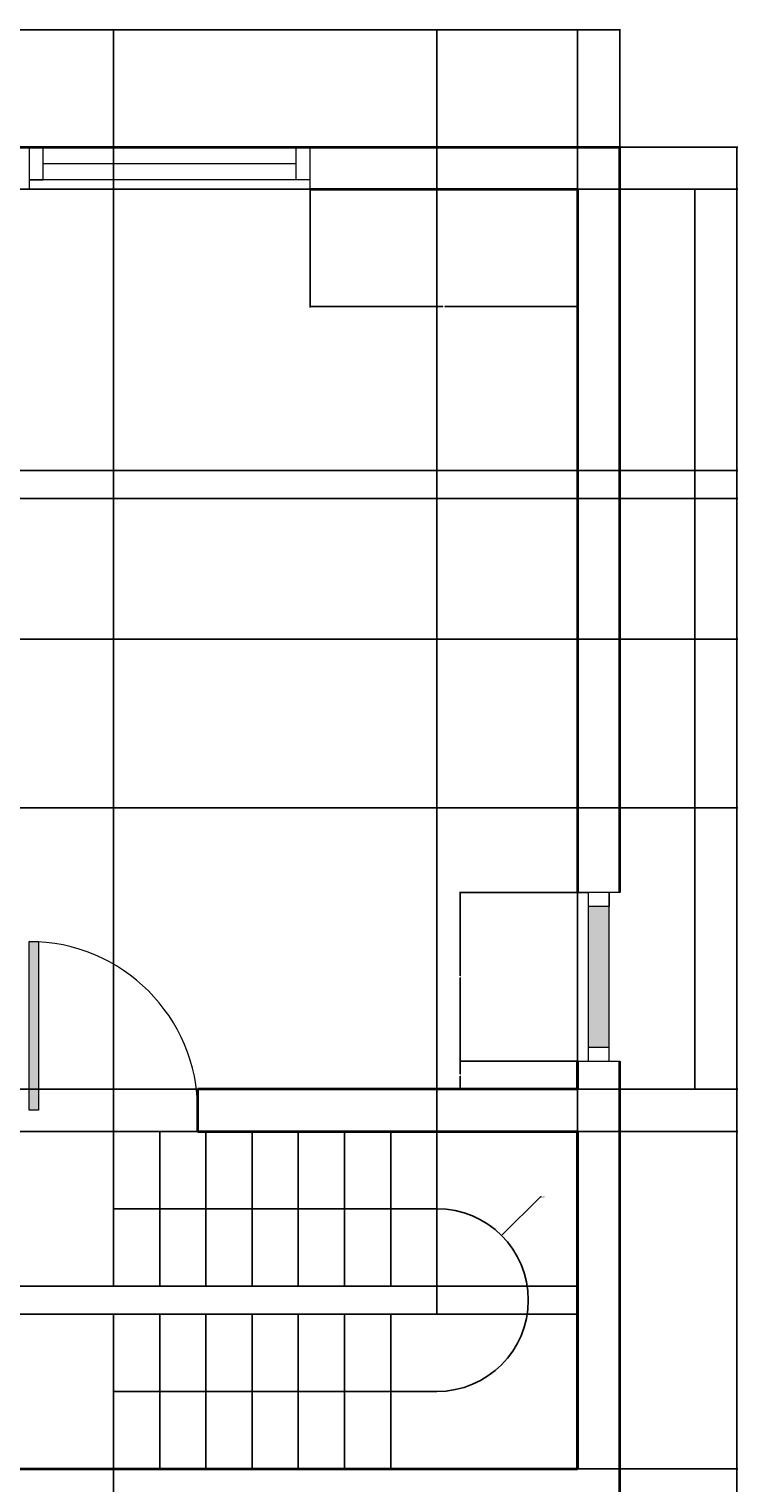
# Model space of a CAD drawing. Units: inches. Extents: x 2039 to 2485, y 1453 to 1986.
# Tile 4 of 4: x 2334 to 2485, y 1676 to 1986. Entities that reach past the tile are written whole.
import ezdxf

# ---------------------------------------------------------------- set-up
doc = ezdxf.new("R2010")
doc.units = ezdxf.units.IN
for name, color, linetype, lineweight in [('A-ANNO-DIMS', 2, 'Continuous', 18), ('A-DOOR', 3, 'Continuous', 18), ('A-FLOR-STRS', 7, 'Continuous', 25), ('A-FLOR-STRS-PNTS', 8, 'Continuous', 13), ('A-GLAZ', 4, 'Continuous', 18), ('A-WALL', 7, 'Continuous', 35)]:
    doc.layers.add(name, color=color, linetype=linetype, lineweight=lineweight)
doc.layers.add('A-OPEN-PATT', color=18, linetype='Continuous', lineweight=13, true_color=0x000000)
doc.styles.get("Standard").update_dxf_attribs({"font": 'arial.ttf'})
doc.dimstyles.get("Standard").update_dxf_attribs({"dimtxt": 0.18, "dimasz": 0.18, "dimexe": 0.18, "dimexo": 0.0625, "dimgap": 0.09, "dimtad": 0, "dimtih": 1, "dimtoh": 1, "dimdec": 4, "dimzin": 0, "dimdsep": 46, "dimtxsty": 'Standard', "dimcen": 0.09, "dimadec": 0, "dimazin": 0, "dimtfac": 1, "dimtdec": 4, "dimtofl": 0, "dimtmove": 0, "dimatfit": 3, "dimfxl": 1, "dimtolj": 1, "dimtzin": 0, "dimarcsym": 0})

# ---------------------------------------------------------------- blocks, each defined once
blk = doc.blocks.new('DOOR-SWING-36IN')
for p, q in [((0, 0), (0, 36)), ((0, 36), (2, 36)), ((2, 36), (2, 0)), ((2, 0), (0, 0))]:
    blk.add_line(p, q)
blk.add_arc((0, 0), 36, 0, 90)
blk = doc.blocks.new('WIN-60IN')
for p, q in [((0, 0), (0, 9)), ((0, 9), (60, 9)), ((3, 2), (3, 9)), ((57, 2), (57, 9)), ((60, 9), (60, 0)), ((57, 5.5), (3, 5.5)), ((0, 2), (60, 2)), ((0, 0), (0, 2)), ((60, 2), (57, 2))]:
    blk.add_line(p, q)
blk = doc.blocks.new('*D16')
at = {"layer": 'A-ANNO-DIMS', "color": 0, "lineweight": -2, "transparency": 16777216}
for p, q in [((2064, 1961.12), (2064, 1986.25)), ((2064.18, 1986.07), (2261.71, 1986.07)), ((2459.82, 1986.07), (2262.29, 1986.07)), ((2460, 1961.12), (2460, 1986.25))]:
    blk.add_line(p, q, dxfattribs=at)
at = {"layer": 'A-ANNO-DIMS', "color": 0, "transparency": 16777216}
for points in [[(2064.18, 1986.1), (2064.18, 1986.04), (2064, 1986.07)], [(2459.82, 1986.1), (2459.82, 1986.04), (2460, 1986.07)]]:
    blk.add_solid(points, dxfattribs=at)
at = {"layer": 'Defpoints', "color": 0, "transparency": 16777216}
for p in [(2460, 1986.07), (2064, 1961.06), (2460, 1961.06)]:
    blk.add_point(p, dxfattribs=at)
at = {"layer": 'A-ANNO-DIMS', "color": 0, "transparency": 16777216, "insert": (2262, 1986.07), "char_height": 0.18, "attachment_point": 5}
blk.add_mtext('\\A1;396', dxfattribs=at)
blk = doc.blocks.new('*D17')
at = {"layer": 'A-ANNO-DIMS', "color": 0, "lineweight": -2, "transparency": 16777216}
for p, q in [((2460.06, 1961.06), (2485.19, 1961.06)), ((2485.01, 1960.88), (2485.01, 1719.74)), ((2485.01, 1478.24), (2485.01, 1719.37)), ((2460.06, 1478.06), (2485.19, 1478.06))]:
    blk.add_line(p, q, dxfattribs=at)
at = {"layer": 'A-ANNO-DIMS', "color": 0, "transparency": 16777216}
for points in [[(2484.98, 1960.88), (2485.04, 1960.88), (2485.01, 1961.06)], [(2484.98, 1478.24), (2485.04, 1478.24), (2485.01, 1478.06)]]:
    blk.add_solid(points, dxfattribs=at)
at = {"layer": 'Defpoints', "color": 0, "transparency": 16777216}
for p in [(2460, 1961.06), (2460, 1478.06), (2485.01, 1478.06)]:
    blk.add_point(p, dxfattribs=at)
at = {"layer": 'A-ANNO-DIMS', "color": 0, "transparency": 16777216, "insert": (2485.01, 1719.56), "char_height": 0.18, "attachment_point": 5}
blk.add_mtext('\\A1;483', dxfattribs=at)
blk = doc.blocks.new('*D19')
at = {"layer": 'A-ANNO-DIMS', "color": 0, "lineweight": -2, "transparency": 16777216}
for p, q in [((2394, 1951.99), (2394, 1926.87)), ((2451, 1951.99), (2451, 1926.87)), ((2394.18, 1927.05), (2422.28, 1927.05)), ((2450.82, 1927.05), (2422.72, 1927.05))]:
    blk.add_line(p, q, dxfattribs=at)
at = {"layer": 'A-ANNO-DIMS', "color": 0, "transparency": 16777216}
for points in [[(2394.18, 1927.08), (2394.18, 1927.02), (2394, 1927.05)], [(2450.82, 1927.08), (2450.82, 1927.02), (2451, 1927.05)]]:
    blk.add_solid(points, dxfattribs=at)
at = {"layer": 'Defpoints', "color": 0, "transparency": 16777216}
for p in [(2394, 1952.06), (2451, 1952.06), (2394, 1927.05)]:
    blk.add_point(p, dxfattribs=at)
at = {"layer": 'A-ANNO-DIMS', "color": 0, "transparency": 16777216, "insert": (2422.5, 1927.05), "char_height": 0.18, "attachment_point": 5}
blk.add_mtext('\\A1;57', dxfattribs=at)
blk = doc.blocks.new('*D32')
at = {"layer": 'A-ANNO-DIMS', "color": 0, "lineweight": -2, "transparency": 16777216}
for p, q in [((2450.94, 1766.06), (2425.81, 1766.06)), ((2425.99, 1765.88), (2425.99, 1763.24)), ((2425.99, 1760.24), (2425.99, 1762.87)), ((2450.94, 1760.06), (2425.81, 1760.06))]:
    blk.add_line(p, q, dxfattribs=at)
at = {"layer": 'A-ANNO-DIMS', "color": 0, "transparency": 16777216}
for points in [[(2425.96, 1765.88), (2426.02, 1765.88), (2425.99, 1766.06)], [(2425.96, 1760.24), (2426.02, 1760.24), (2425.99, 1760.06)]]:
    blk.add_solid(points, dxfattribs=at)
at = {"layer": 'Defpoints', "color": 0, "transparency": 16777216}
for p in [(2425.99, 1766.06), (2451, 1766.06), (2451, 1760.06)]:
    blk.add_point(p, dxfattribs=at)
at = {"layer": 'A-ANNO-DIMS', "color": 0, "transparency": 16777216, "insert": (2425.99, 1763.06), "char_height": 0.18, "attachment_point": 5}
blk.add_mtext('\\A1;6', dxfattribs=at)
blk = doc.blocks.new('*D33')
at = {"layer": 'A-ANNO-DIMS', "color": 0, "lineweight": -2, "transparency": 16777216}
for p, q in [((2450.94, 1802.06), (2425.81, 1802.06)), ((2425.99, 1801.88), (2425.99, 1784.24)), ((2425.99, 1766.24), (2425.99, 1783.87)), ((2450.94, 1766.06), (2425.81, 1766.06))]:
    blk.add_line(p, q, dxfattribs=at)
at = {"layer": 'A-ANNO-DIMS', "color": 0, "transparency": 16777216}
for points in [[(2425.96, 1801.88), (2426.02, 1801.88), (2425.99, 1802.06)], [(2425.96, 1766.24), (2426.02, 1766.24), (2425.99, 1766.06)]]:
    blk.add_solid(points, dxfattribs=at)
at = {"layer": 'Defpoints', "color": 0, "transparency": 16777216}
for p in [(2425.99, 1802.06), (2451, 1802.06), (2451, 1766.06)]:
    blk.add_point(p, dxfattribs=at)
at = {"layer": 'A-ANNO-DIMS', "color": 0, "transparency": 16777216, "insert": (2425.99, 1784.06), "char_height": 0.18, "attachment_point": 5}
blk.add_mtext('\\A1;36', dxfattribs=at)
blk = doc.blocks.new('*D37')
at = {"layer": 'A-ANNO-DIMS', "color": 0, "lineweight": -2, "transparency": 16777216}
for p, q in [((2451.06, 1952.06), (2476.19, 1952.06)), ((2476.01, 1951.88), (2476.01, 1856.24)), ((2476.01, 1760.24), (2476.01, 1855.87)), ((2451.06, 1760.06), (2476.19, 1760.06))]:
    blk.add_line(p, q, dxfattribs=at)
at = {"layer": 'A-ANNO-DIMS', "color": 0, "transparency": 16777216}
for points in [[(2475.98, 1951.88), (2476.04, 1951.88), (2476.01, 1952.06)], [(2475.98, 1760.24), (2476.04, 1760.24), (2476.01, 1760.06)]]:
    blk.add_solid(points, dxfattribs=at)
at = {"layer": 'Defpoints', "color": 0, "transparency": 16777216}
for p in [(2451, 1952.06), (2451, 1760.06), (2476.01, 1760.06)]:
    blk.add_point(p, dxfattribs=at)
at = {"layer": 'A-ANNO-DIMS', "color": 0, "transparency": 16777216, "insert": (2476.01, 1856.06), "char_height": 0.18, "attachment_point": 5}
blk.add_mtext('\\A1;192', dxfattribs=at)
blk = doc.blocks.new('*D46')
at = {"layer": 'A-ANNO-DIMS', "color": 0, "lineweight": -2, "transparency": 16777216}
for p, q in [((2322.06, 1952.06), (2485.19, 1952.06)), ((2485.01, 1951.88), (2485.01, 1922.24)), ((2485.01, 1892.24), (2485.01, 1921.87)), ((2322.06, 1892.06), (2485.19, 1892.06))]:
    blk.add_line(p, q, dxfattribs=at)
at = {"layer": 'A-ANNO-DIMS', "color": 0, "transparency": 16777216}
for points in [[(2484.98, 1951.88), (2485.04, 1951.88), (2485.01, 1952.06)], [(2484.98, 1892.24), (2485.04, 1892.24), (2485.01, 1892.06)]]:
    blk.add_solid(points, dxfattribs=at)
at = {"layer": 'Defpoints', "color": 0, "transparency": 16777216}
for p in [(2322, 1952.06), (2485.01, 1952.06), (2322, 1892.06)]:
    blk.add_point(p, dxfattribs=at)
at = {"layer": 'A-ANNO-DIMS', "color": 0, "transparency": 16777216, "insert": (2485.01, 1922.06), "char_height": 0.18, "attachment_point": 5}
blk.add_mtext('\\A1;60', dxfattribs=at)
blk = doc.blocks.new('*D48')
at = {"layer": 'A-ANNO-DIMS', "color": 0, "lineweight": -2, "transparency": 16777216}
for p, q in [((2322.06, 1820.06), (2485.19, 1820.06)), ((2485.01, 1819.88), (2485.01, 1790.24)), ((2485.01, 1760.24), (2485.01, 1789.87)), ((2322.06, 1760.06), (2485.19, 1760.06))]:
    blk.add_line(p, q, dxfattribs=at)
at = {"layer": 'A-ANNO-DIMS', "color": 0, "transparency": 16777216}
for points in [[(2484.98, 1819.88), (2485.04, 1819.88), (2485.01, 1820.06)], [(2484.98, 1760.24), (2485.04, 1760.24), (2485.01, 1760.06)]]:
    blk.add_solid(points, dxfattribs=at)
at = {"layer": 'Defpoints', "color": 0, "transparency": 16777216}
for p in [(2322, 1820.06), (2485.01, 1820.06), (2322, 1760.06)]:
    blk.add_point(p, dxfattribs=at)
at = {"layer": 'A-ANNO-DIMS', "color": 0, "transparency": 16777216, "insert": (2485.01, 1790.06), "char_height": 0.18, "attachment_point": 5}
blk.add_mtext('\\A1;60', dxfattribs=at)
blk = doc.blocks.new('*D50')
at = {"layer": 'A-ANNO-DIMS', "color": 0, "lineweight": -2, "transparency": 16777216}
for p, q in [((2322.06, 1892.06), (2485.19, 1892.06)), ((2485.01, 1891.88), (2485.01, 1889.24)), ((2322.06, 1886.06), (2485.19, 1886.06)), ((2485.01, 1886.24), (2485.01, 1888.87))]:
    blk.add_line(p, q, dxfattribs=at)
at = {"layer": 'A-ANNO-DIMS', "color": 0, "transparency": 16777216}
for points in [[(2484.98, 1891.88), (2485.04, 1891.88), (2485.01, 1892.06)], [(2484.98, 1886.24), (2485.04, 1886.24), (2485.01, 1886.06)]]:
    blk.add_solid(points, dxfattribs=at)
at = {"layer": 'Defpoints', "color": 0, "transparency": 16777216}
for p in [(2322, 1892.06), (2485.01, 1892.06), (2322, 1886.06)]:
    blk.add_point(p, dxfattribs=at)
at = {"layer": 'A-ANNO-DIMS', "color": 0, "transparency": 16777216, "insert": (2485.01, 1889.06), "char_height": 0.18, "attachment_point": 5}
blk.add_mtext('\\A1;6', dxfattribs=at)
blk = doc.blocks.new('*D53')
at = {"layer": 'A-ANNO-DIMS', "color": 0, "lineweight": -2, "transparency": 16777216}
for p, q in [((2322.06, 1886.06), (2485.19, 1886.06)), ((2485.01, 1885.88), (2485.01, 1871.24)), ((2485.01, 1856.24), (2485.01, 1870.87)), ((2331.06, 1856.06), (2485.19, 1856.06))]:
    blk.add_line(p, q, dxfattribs=at)
at = {"layer": 'A-ANNO-DIMS', "color": 0, "transparency": 16777216}
for points in [[(2484.98, 1885.88), (2485.04, 1885.88), (2485.01, 1886.06)], [(2484.98, 1856.24), (2485.04, 1856.24), (2485.01, 1856.06)]]:
    blk.add_solid(points, dxfattribs=at)
at = {"layer": 'Defpoints', "color": 0, "transparency": 16777216}
for p in [(2322, 1886.06), (2485.01, 1886.06), (2331, 1856.06)]:
    blk.add_point(p, dxfattribs=at)
at = {"layer": 'A-ANNO-DIMS', "color": 0, "transparency": 16777216, "insert": (2485.01, 1871.06), "char_height": 0.18, "attachment_point": 5}
blk.add_mtext('\\A1;30', dxfattribs=at)
blk = doc.blocks.new('*D56')
at = {"layer": 'A-ANNO-DIMS', "color": 0, "lineweight": -2, "transparency": 16777216}
for p, q in [((2286.06, 1760.06), (2485.19, 1760.06)), ((2485.01, 1759.88), (2485.01, 1755.74)), ((2485.01, 1751.24), (2485.01, 1755.37)), ((2286.06, 1751.06), (2485.19, 1751.06))]:
    blk.add_line(p, q, dxfattribs=at)
at = {"layer": 'A-ANNO-DIMS', "color": 0, "transparency": 16777216}
for points in [[(2484.98, 1759.88), (2485.04, 1759.88), (2485.01, 1760.06)], [(2484.98, 1751.24), (2485.04, 1751.24), (2485.01, 1751.06)]]:
    blk.add_solid(points, dxfattribs=at)
at = {"layer": 'Defpoints', "color": 0, "transparency": 16777216}
for p in [(2286, 1760.06), (2485.01, 1760.06), (2286, 1751.06)]:
    blk.add_point(p, dxfattribs=at)
at = {"layer": 'A-ANNO-DIMS', "color": 0, "transparency": 16777216, "insert": (2485.01, 1755.56), "char_height": 0.18, "attachment_point": 5}
blk.add_mtext('\\A1;9', dxfattribs=at)
blk = doc.blocks.new('*D57')
at = {"layer": 'A-ANNO-DIMS', "color": 0, "lineweight": -2, "transparency": 16777216}
for p, q in [((2451.06, 1751.06), (2485.19, 1751.06)), ((2485.01, 1750.88), (2485.01, 1715.24)), ((2485.01, 1679.24), (2485.01, 1714.88)), ((2451.06, 1679.06), (2485.19, 1679.06))]:
    blk.add_line(p, q, dxfattribs=at)
at = {"layer": 'A-ANNO-DIMS', "color": 0, "transparency": 16777216}
for points in [[(2484.98, 1750.88), (2485.04, 1750.88), (2485.01, 1751.06)], [(2484.98, 1679.24), (2485.04, 1679.24), (2485.01, 1679.06)]]:
    blk.add_solid(points, dxfattribs=at)
at = {"layer": 'Defpoints', "color": 0, "transparency": 16777216}
for p in [(2451, 1751.06), (2485.01, 1751.06), (2451, 1679.06)]:
    blk.add_point(p, dxfattribs=at)
at = {"layer": 'A-ANNO-DIMS', "color": 0, "transparency": 16777216, "insert": (2485.01, 1715.06), "char_height": 0.18, "attachment_point": 5}
blk.add_mtext('\\A1;72', dxfattribs=at)
blk = doc.blocks.new('*D58')
at = {"layer": 'A-ANNO-DIMS', "color": 0, "lineweight": -2, "transparency": 16777216}
for p, q in [((2331, 1678.99), (2331, 1452.87)), ((2352, 1678.99), (2352, 1452.87)), ((2331.18, 1453.05), (2341.3, 1453.05)), ((2351.82, 1453.05), (2341.71, 1453.05))]:
    blk.add_line(p, q, dxfattribs=at)
at = {"layer": 'A-ANNO-DIMS', "color": 0, "transparency": 16777216}
for points in [[(2331.18, 1453.08), (2331.18, 1453.02), (2331, 1453.05)], [(2351.82, 1453.08), (2351.82, 1453.02), (2352, 1453.05)]]:
    blk.add_solid(points, dxfattribs=at)
at = {"layer": 'Defpoints', "color": 0, "transparency": 16777216}
for p in [(2331, 1679.06), (2352, 1679.06), (2352, 1453.05)]:
    blk.add_point(p, dxfattribs=at)
at = {"layer": 'A-ANNO-DIMS', "color": 0, "transparency": 16777216, "insert": (2341.5, 1453.05), "char_height": 0.18, "attachment_point": 5}
blk.add_mtext('\\A1;21', dxfattribs=at)
blk = doc.blocks.new('*D59')
at = {"layer": 'A-ANNO-DIMS', "color": 0, "lineweight": -2, "transparency": 16777216}
for p, q in [((2352, 1751.12), (2352, 1986.25)), ((2352.18, 1986.07), (2386.28, 1986.07)), ((2420.82, 1986.07), (2386.72, 1986.07)), ((2421, 1751.12), (2421, 1986.25))]:
    blk.add_line(p, q, dxfattribs=at)
at = {"layer": 'A-ANNO-DIMS', "color": 0, "transparency": 16777216}
for points in [[(2352.18, 1986.1), (2352.18, 1986.04), (2352, 1986.07)], [(2420.82, 1986.1), (2420.82, 1986.04), (2421, 1986.07)]]:
    blk.add_solid(points, dxfattribs=at)
at = {"layer": 'Defpoints', "color": 0, "transparency": 16777216}
for p in [(2421, 1986.07), (2352, 1751.06), (2421, 1751.06)]:
    blk.add_point(p, dxfattribs=at)
at = {"layer": 'A-ANNO-DIMS', "color": 0, "transparency": 16777216, "insert": (2386.5, 1986.07), "char_height": 0.18, "attachment_point": 5}
blk.add_mtext('\\A1;69', dxfattribs=at)
blk = doc.blocks.new('*D60')
at = {"layer": 'A-ANNO-DIMS', "color": 0, "lineweight": -2, "transparency": 16777216}
for p, q in [((2421, 1751.12), (2421, 1986.25)), ((2421.18, 1986.07), (2435.78, 1986.07)), ((2450.82, 1986.07), (2436.22, 1986.07)), ((2451, 1751.12), (2451, 1986.25))]:
    blk.add_line(p, q, dxfattribs=at)
at = {"layer": 'A-ANNO-DIMS', "color": 0, "transparency": 16777216}
for points in [[(2421.18, 1986.1), (2421.18, 1986.04), (2421, 1986.07)], [(2450.82, 1986.1), (2450.82, 1986.04), (2451, 1986.07)]]:
    blk.add_solid(points, dxfattribs=at)
at = {"layer": 'Defpoints', "color": 0, "transparency": 16777216}
for p in [(2451, 1986.07), (2421, 1751.06), (2451, 1751.06)]:
    blk.add_point(p, dxfattribs=at)
at = {"layer": 'A-ANNO-DIMS', "color": 0, "transparency": 16777216, "insert": (2436, 1986.07), "char_height": 0.18, "attachment_point": 5}
blk.add_mtext('\\A1;30', dxfattribs=at)
blk = doc.blocks.new('*D61')
at = {"layer": 'A-ANNO-DIMS', "color": 0, "lineweight": -2, "transparency": 16777216}
for p, q in [((2351.94, 1751.06), (2038.81, 1751.06)), ((2038.99, 1750.88), (2038.99, 1734.74)), ((2038.99, 1718.24), (2038.99, 1734.37)), ((2351.94, 1718.06), (2038.81, 1718.06))]:
    blk.add_line(p, q, dxfattribs=at)
at = {"layer": 'A-ANNO-DIMS', "color": 0, "transparency": 16777216}
for points in [[(2038.96, 1750.88), (2039.02, 1750.88), (2038.99, 1751.06)], [(2038.96, 1718.24), (2039.02, 1718.24), (2038.99, 1718.06)]]:
    blk.add_solid(points, dxfattribs=at)
at = {"layer": 'Defpoints', "color": 0, "transparency": 16777216}
for p in [(2038.99, 1751.06), (2352, 1751.06), (2352, 1718.06)]:
    blk.add_point(p, dxfattribs=at)
at = {"layer": 'A-ANNO-DIMS', "color": 0, "transparency": 16777216, "insert": (2038.99, 1734.56), "char_height": 0.18, "attachment_point": 5}
blk.add_mtext('\\A1;33', dxfattribs=at)
blk = doc.blocks.new('*D62')
at = {"layer": 'A-ANNO-DIMS', "color": 0, "lineweight": -2, "transparency": 16777216}
for p, q in [((2351.94, 1718.06), (2038.81, 1718.06)), ((2038.99, 1717.88), (2038.99, 1715.24)), ((2038.99, 1712.24), (2038.99, 1714.87)), ((2351.94, 1712.06), (2038.81, 1712.06))]:
    blk.add_line(p, q, dxfattribs=at)
at = {"layer": 'A-ANNO-DIMS', "color": 0, "transparency": 16777216}
for points in [[(2038.96, 1717.88), (2039.02, 1717.88), (2038.99, 1718.06)], [(2038.96, 1712.24), (2039.02, 1712.24), (2038.99, 1712.06)]]:
    blk.add_solid(points, dxfattribs=at)
at = {"layer": 'Defpoints', "color": 0, "transparency": 16777216}
for p in [(2038.99, 1718.06), (2352, 1718.06), (2352, 1712.06)]:
    blk.add_point(p, dxfattribs=at)
at = {"layer": 'A-ANNO-DIMS', "color": 0, "transparency": 16777216, "insert": (2038.99, 1715.06), "char_height": 0.18, "attachment_point": 5}
blk.add_mtext('\\A1;6', dxfattribs=at)
blk = doc.blocks.new('*D65')
at = {"layer": 'A-ANNO-DIMS', "color": 0, "lineweight": -2, "transparency": 16777216}
for p, q in [((2451.06, 1679.06), (2485.19, 1679.06)), ((2485.01, 1678.88), (2485.01, 1676.24)), ((2485.01, 1673.24), (2485.01, 1675.87)), ((2451.06, 1673.06), (2485.19, 1673.06))]:
    blk.add_line(p, q, dxfattribs=at)
at = {"layer": 'A-ANNO-DIMS', "color": 0, "transparency": 16777216}
for points in [[(2484.98, 1678.88), (2485.04, 1678.88), (2485.01, 1679.06)], [(2484.98, 1673.24), (2485.04, 1673.24), (2485.01, 1673.06)]]:
    blk.add_solid(points, dxfattribs=at)
at = {"layer": 'Defpoints', "color": 0, "transparency": 16777216}
for p in [(2451, 1679.06), (2485.01, 1679.06), (2451, 1673.06)]:
    blk.add_point(p, dxfattribs=at)
at = {"layer": 'A-ANNO-DIMS', "color": 0, "transparency": 16777216, "insert": (2485.01, 1676.06), "char_height": 0.18, "attachment_point": 5}
blk.add_mtext('\\A1;6', dxfattribs=at)
blk = doc.blocks.new('*D69')
at = {"layer": 'A-ANNO-DIMS', "color": 0, "lineweight": -2, "transparency": 16777216}
for p, q in [((2443.07, 1737.11), (2434.92, 1728.97)), ((2443.25, 1737.11), (2443.07, 1737.11)), ((2420.91, 1715.06), (2421.09, 1715.06)), ((2421, 1714.97), (2421, 1715.15))]:
    blk.add_line(p, q, dxfattribs=at)
at = {"layer": 'A-ANNO-DIMS', "color": 0, "transparency": 16777216}
blk.add_solid([(2434.9, 1728.99), (2434.94, 1728.95), (2434.79, 1728.84)], dxfattribs=at)
at = {"layer": 'Defpoints', "color": 0, "transparency": 16777216}
for p in [(2434.79, 1728.84), (2421, 1715.06)]:
    blk.add_point(p, dxfattribs=at)
at = {"layer": 'A-ANNO-DIMS', "color": 0, "transparency": 16777216, "insert": (2443.66, 1737.11), "char_height": 0.18, "attachment_point": 5}
blk.add_mtext('\\A1;R19.5', dxfattribs=at)

msp = doc.modelspace()

# ---------------------------------------------------------------- hatches: boundary and pattern name
at = {"layer": 'A-OPEN-PATT'}
h = msp.add_hatch(color=256, dxfattribs=at)
h.dxf.hatch_style = 1
h.paths.add_polyline_path([(2070.75, 1853.06), (2066.25, 1853.06), (2066.25, 1799.06), (2070.75, 1799.06)])
h.paths.add_polyline_path([(2080, 1791.5, 0.013897), (2078, 1791.56), (2078, 1755.56), (2080, 1755.56)])
h.paths.add_polyline_path([(2070.75, 1712.06), (2066.25, 1712.06), (2066.25, 1670.06), (2070.75, 1670.06)])
h.paths.add_polyline_path([(2070.75, 1568.06), (2066.25, 1568.06), (2066.25, 1526.06), (2070.75, 1526.06)])
h.paths.add_polyline_path([(2080, 1518.5, 0.013897), (2078, 1518.56), (2078, 1482.56), (2080, 1482.56)])
h.paths.add_polyline_path([(2362.5, 1666.06), (2326.5, 1666.06), (2326.5, 1664.06), (2362.45, 1664.06, 0.013897)])
h.paths.add_polyline_path([(2457.75, 1601.06), (2453.25, 1601.06), (2453.25, 1553.06), (2457.75, 1553.06)])
h.paths.add_polyline_path([(2457.75, 1799.06), (2453.25, 1799.06), (2453.25, 1769.06), (2457.75, 1769.06)])
h.paths.add_polyline_path([(2336, 1791.5, 0.013897), (2334, 1791.56), (2334, 1755.56), (2336, 1755.56)])
h.paths.add_polyline_path([(2255, 1788.5, 0.015162), (2253, 1788.56), (2253, 1755.56), (2255, 1755.56)])
h.paths.add_polyline_path([(2331, 1830.06), (2322, 1830.06), (2322, 1828.06), (2331, 1828.06)])
h.paths.add_polyline_path([(2250, 1896.06), (2245.5, 1896.06), (2241, 1896.06), (2241, 1894.06), (2250, 1894.06)])
h.paths.add_polyline_path([(2271.5, 1896.06), (2250, 1896.06), (2250, 1894.06), (2271.5, 1894.06)])
h.paths.add_polyline_path([(2304, 1958.81), (2268, 1958.81), (2268, 1954.31), (2304, 1954.31)])

# ---------------------------------------------------------------- linework, layer by layer
at = {"layer": 'A-FLOR-STRS'}
for p, q in [((2352, 1751.06), (2421, 1751.06)), ((2352, 1751.06), (2352, 1718.06)), ((2361.86, 1751.06), (2361.86, 1718.06)), ((2421, 1751.06), (2370, 1751.06)), ((2371.72, 1751.06), (2371.72, 1718.06)), ((2381.57, 1751.06), (2381.57, 1718.06)), ((2391.43, 1751.06), (2391.43, 1718.06)), ((2401.29, 1751.06), (2401.29, 1718.06)), ((2411.15, 1751.06), (2411.15, 1718.06)), ((2451, 1751.06), (2421, 1751.06)), ((2421, 1751.06), (2421, 1712.06)), ((2421, 1718.06), (2421, 1751.06)), ((2421, 1734.56), (2352, 1734.56)), ((2451, 1718.06), (2352, 1718.06)), ((2451, 1712.06), (2352, 1712.06)), ((2352, 1712.06), (2352, 1679.06)), ((2361.86, 1712.06), (2361.86, 1679.06)), ((2371.72, 1712.06), (2371.72, 1679.06)), ((2381.57, 1712.06), (2381.57, 1679.06)), ((2391.43, 1712.06), (2391.43, 1679.06)), ((2401.29, 1712.06), (2401.29, 1679.06)), ((2411.15, 1712.06), (2411.15, 1679.06)), ((2421, 1695.56), (2352, 1695.56))]:
    msp.add_line(p, q, dxfattribs=at)
msp.add_arc((2421, 1715.06), 19.5, 270, 90, dxfattribs=at)
at = {"layer": 'A-FLOR-STRS-PNTS'}
for p in [(2361.86, 1751.06), (2371.72, 1751.06), (2381.57, 1751.06), (2391.43, 1751.06), (2401.29, 1751.06), (2411.15, 1751.06)]:
    msp.add_point(p, dxfattribs=at)
at = {"layer": 'A-GLAZ'}
for p, q in [((2337, 1961.06), (2391, 1961.06)), ((2391, 1954.06), (2391, 1957.56)), ((2460, 1802.06), (2451, 1802.06)), ((2451, 1802.06), (2453.25, 1802.06)), ((2453.25, 1802.06), (2453.25, 1766.06)), ((2457.75, 1766.06), (2457.75, 1802.06)), ((2457.75, 1802.06), (2457.75, 1799.06)), ((2457.75, 1799.06), (2453.25, 1799.06)), ((2453.25, 1799.06), (2453.25, 1769.06)), ((2453.25, 1769.06), (2457.75, 1769.06)), ((2451, 1766.06), (2460, 1766.06)), ((2453.25, 1766.06), (2457.75, 1766.06))]:
    msp.add_line(p, q, dxfattribs=at)
at = {"layer": 'A-WALL'}
for p, q in [((2331, 1961.06), (2451, 1961.06)), ((2451, 1961.06), (2460, 1961.06)), ((2460, 1802.06), (2460, 1961.06)), ((2394, 1952.06), (2451, 1952.06)), ((2451, 1952.06), (2451, 1802.06)), ((2451, 1765.06), (2451, 1766.06)), ((2451, 1766.06), (2451, 1760.06)), ((2451, 1760.06), (2451, 1765.06)), ((2460, 1751.06), (2460, 1766.06)), ((2451, 1760.06), (2370, 1760.06)), ((2370, 1751.06), (2370, 1760.06)), ((2370, 1751.06), (2451, 1751.06)), ((2451, 1679.06), (2451, 1751.06)), ((2451, 1751.06), (2451, 1679.06)), ((2460, 1604.06), (2460, 1751.06)), ((2451, 1679.06), (2451, 1715.06)), ((2331, 1679.06), (2451, 1679.06))]:
    msp.add_line(p, q, dxfattribs=at)

# ---------------------------------------------------------------- block references
at = {"layer": 'A-DOOR'}
msp.add_blockref('DOOR-SWING-36IN', (2334, 1755.56), dxfattribs=at)
at = {"layer": 'A-GLAZ', "extrusion": (0, 0, -1), "zscale": -1}
msp.add_blockref('WIN-60IN', (-2394, 1952.06), dxfattribs=at)

# ---------------------------------------------------------------- dimensions: what is measured, and where the dimension line sits
at = {"layer": 'A-ANNO-DIMS'}
for base, p1, p2, picture, middle in [((2460, 1986.07), (2064, 1961.06), (2460, 1961.06), '*D16', (2262, 1986.07)), ((2421, 1986.07), (2352, 1751.06), (2421, 1751.06), '*D59', (2386.5, 1986.07)), ((2451, 1986.07), (2421, 1751.06), (2451, 1751.06), '*D60', (2436, 1986.07)), ((2352, 1453.05), (2331, 1679.06), (2352, 1679.06), '*D58', (2341.5, 1453.05))]:
    dim = msp.add_linear_dim(base=base, p1=p1, p2=p2, dimstyle='Standard', override={"dimdec": 0, "dimlfac": 1, "dimrnd": 0, "dimzin": 0, "dimdsep": 46, "dimlunit": 2}, dxfattribs=at)
    dim.commit()
    dim.dimension.update_dxf_attribs({"geometry": picture, "text_midpoint": middle})
for base, p1, p2, angle, picture, middle in [((2485.01, 1478.06), (2460, 1961.06), (2460, 1478.06), 270, '*D17', (2485.01, 1719.56)), ((2485.01, 1952.06), (2322, 1892.06), (2322, 1952.06), 90, '*D46', (2485.01, 1922.06)), ((2394, 1927.05), (2451, 1952.06), (2394, 1952.06), 180, '*D19', (2422.5, 1927.05)), ((2476.01, 1760.06), (2451, 1952.06), (2451, 1760.06), 270, '*D37', (2476.01, 1856.06)), ((2485.01, 1892.06), (2322, 1886.06), (2322, 1892.06), 90, '*D50', (2485.01, 1889.06)), ((2485.01, 1886.06), (2331, 1856.06), (2322, 1886.06), 90, '*D53', (2485.01, 1871.06)), ((2485.01, 1820.06), (2322, 1760.06), (2322, 1820.06), 90, '*D48', (2485.01, 1790.06)), ((2425.99, 1802.06), (2451, 1766.06), (2451, 1802.06), 90, '*D33', (2425.99, 1784.06)), ((2425.99, 1766.06), (2451, 1760.06), (2451, 1766.06), 90, '*D32', (2425.99, 1763.06)), ((2485.01, 1760.06), (2286, 1751.06), (2286, 1760.06), 90, '*D56', (2485.01, 1755.56)), ((2038.99, 1751.06), (2352, 1718.06), (2352, 1751.06), 90, '*D61', (2038.99, 1734.56)), ((2485.01, 1751.06), (2451, 1679.06), (2451, 1751.06), 90, '*D57', (2485.01, 1715.06)), ((2038.99, 1718.06), (2352, 1712.06), (2352, 1718.06), 90, '*D62', (2038.99, 1715.06)), ((2485.01, 1679.06), (2451, 1673.06), (2451, 1679.06), 90, '*D65', (2485.01, 1676.06))]:
    dim = msp.add_linear_dim(base=base, p1=p1, p2=p2, angle=angle, dimstyle='Standard', override={"dimdec": 0, "dimlfac": 1, "dimrnd": 0, "dimzin": 0, "dimdsep": 46, "dimlunit": 2}, dxfattribs=at)
    dim.commit()
    dim.dimension.update_dxf_attribs({"geometry": picture, "text_midpoint": middle})
dim = msp.add_radius_dim(center=(2421, 1715.06), mpoint=(2434.79, 1728.84), dimstyle='Standard', override={"dimdec": 1, "dimlfac": 1, "dimrnd": 0, "dimzin": 0, "dimdsep": 46, "dimlunit": 2}, dxfattribs=at)
dim.commit()
dim.dimension.update_dxf_attribs({"geometry": '*D69', "text_midpoint": (2443.66, 1737.11), "dimtype": 164})

doc.saveas('drawing.dxf')
